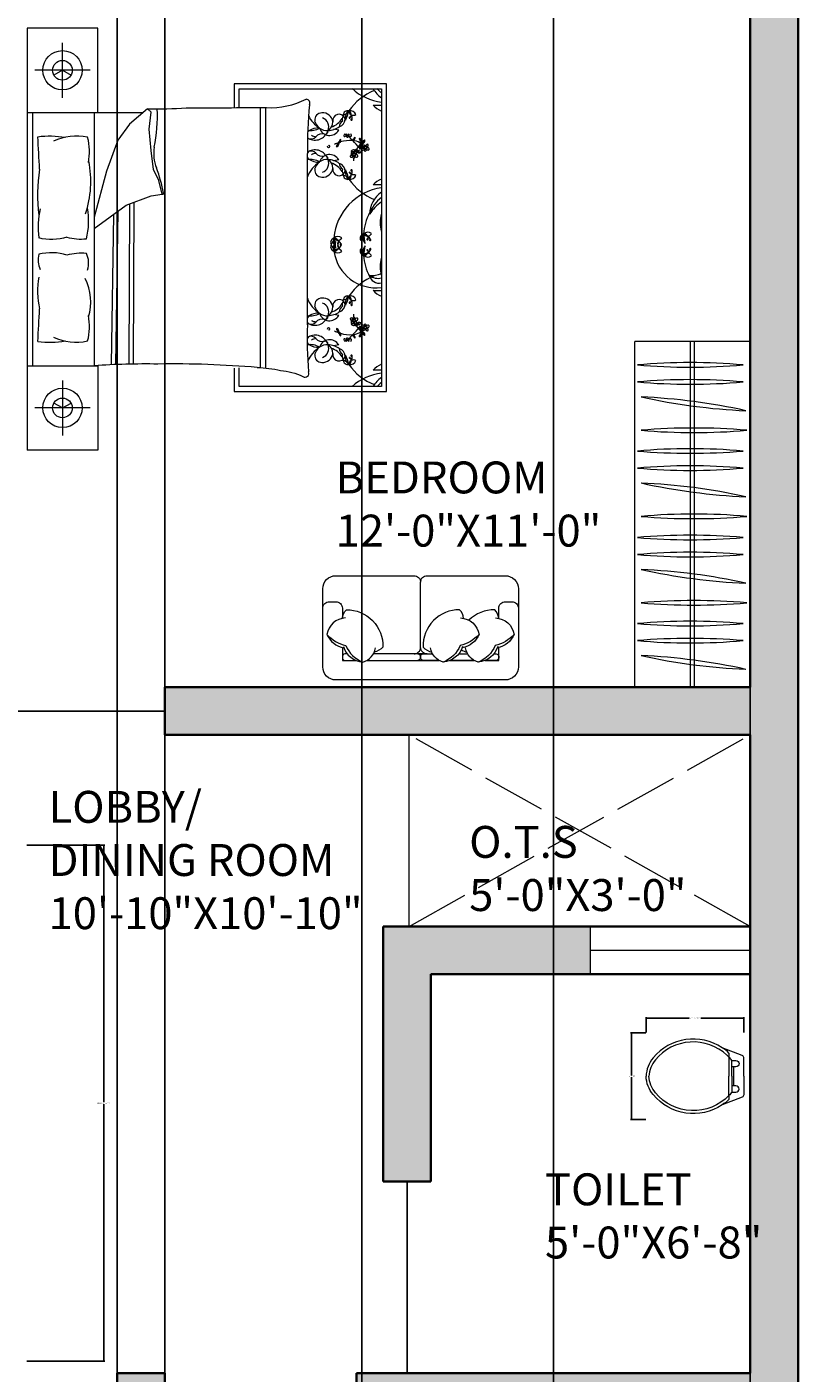
# Model space of a CAD drawing. Units: inches. Extents: x -16 to 587, y -783 to 64.
# Tile 11 of 14: x 92 to 237, y -392 to -138. Entities that reach past the tile are written whole.
import ezdxf

# ---------------------------------------------------------------- set-up
doc = ezdxf.new("R2010")
doc.units = ezdxf.units.IN
doc.header["$MEASUREMENT"] = 0
doc.linetypes.add('ACAD_ISO02W100', pattern=[15, 12, -3])
for name, color, linetype, lineweight in [('A-ANNO-DIMS', 2, 'Continuous', 18), ('A-AREA-IDEN', 7, 'Continuous', 18), ('A-DOOR', 3, 'Continuous', 25), ('A-FLOR-FIXT', 9, 'Continuous', 18), ('A-FLOR-OPEN', 8, 'ACAD_ISO02W100', 13), ('A-FURN', 8, 'Continuous', 18), ('A-GLAZ', 4, 'Continuous', 18), ('A-WALL', 7, 'Continuous', 35), ('A-WALL-PATT', 23, 'Continuous', 13)]:
    doc.layers.add(name, color=color, linetype=linetype, lineweight=lineweight)
doc.styles.get("Standard").update_dxf_attribs({"font": 'arial.ttf'})
doc.dimstyles.get("Standard").update_dxf_attribs({"dimtxt": 0.18, "dimasz": 0.18, "dimexe": 0.18, "dimexo": 0.0625, "dimgap": 0.09, "dimtad": 0, "dimtih": 1, "dimtoh": 1, "dimdec": 0, "dimzin": 0, "dimdsep": 46, "dimlunit": 3, "dimtxsty": 'Standard', "dimcen": 0.09, "dimadec": 0, "dimazin": 0, "dimtfac": 1, "dimtdec": 0, "dimtofl": 0, "dimtmove": 0, "dimatfit": 3, "dimfxl": 1, "dimtolj": 1, "dimtzin": 0, "dimarcsym": 0})

# ---------------------------------------------------------------- blocks, each defined once
blk = doc.blocks.new('BED-DOUBLE-COMPACT')
for p, q in [((0, 79.37), (0, 0)), ((6.61, 66.25), (6.61, 76.62)), ((11.8, 71.43), (1.43, 71.43)), ((38.91, 68.89), (38.91, 64.4)), ((67.5, 68.89), (38.91, 68.89)), ((67.5, 11.03), (67.5, 68.89)), ((39.83, 64.41), (39.83, 67.97)), ((39.83, 67.97), (66.58, 67.97)), ((66.58, 67.97), (66.58, 11.95)), ((0, 63.5), (21.78, 63.5)), ((1.02, 15.87), (1.02, 63.5)), ((12.54, 63.5), (12.54, 15.87)), ((22.61, 64.21), (19.24, 61.31)), ((23.26, 63.56), (22.61, 64.21)), ((22.93, 60.35), (23.26, 63.56)), ((43.86, 15.51), (43.86, 64.41)), ((44.85, 15.44), (44.85, 64.41)), ((19.24, 61.31), (16.99, 58.26)), ((16.99, 58.26), (14.9, 52.47)), ((23.26, 56.33), (22.93, 60.35)), ((58.53, 60.15), (57.63, 60.33)), ((23.74, 52.79), (23.26, 56.33)), ((52.64, 23.57), (52.64, 55.8)), ((58.53, 54.61), (57.63, 54.43)), ((14.9, 52.47), (12.54, 43.82)), ((24.7, 50.7), (23.74, 52.79)), ((25.34, 48.13), (24.7, 50.7)), ((23.26, 47.81), (25.34, 48.13)), ((12.54, 41.69), (18.6, 46.04)), ((18.6, 46.04), (23.26, 47.81)), ((19.15, 16.16), (19.27, 46.3)), ((19.97, 16.15), (20.09, 46.61)), ((15.84, 16.09), (16.24, 44.34)), ((16.65, 16.12), (17.06, 44.94)), ((58.53, 25.32), (57.63, 25.49)), ((58.53, 19.77), (57.63, 19.6)), ((38.91, 15.43), (38.91, 11.03)), ((39.83, 11.95), (39.83, 15.45)), ((6.61, 13.12), (6.61, 2.75)), ((38.91, 11.03), (67.5, 11.03)), ((66.58, 11.95), (39.83, 11.95)), ((11.8, 7.94), (1.43, 7.94))]:
    blk.add_line(p, q)
for points in [[(13.23, 63.5), (13.23, 79.37), (0, 79.37)], [(6.61, 71.43), (5.01, 70.51)], [(6.61, 71.43), (8.22, 70.51)], [(0, 15.87), (13.23, 15.87), (13.23, 0), (0, 0)], [(6.61, 7.94), (5.01, 8.86)], [(6.61, 7.94), (8.22, 8.86)]]:
    blk.add_lwpolyline(points)
for points in [[(29.88, 64.37, -0.001242), (44.94, 64.41, 0.127202), (52.44, 66)], [(1.98, 58.94, -0.074897), (7.16, 58.84, 0.472817)], [(7.45, 40.06, -0.14099), (2.16, 39.9, -0.235245)], [(7.45, 36.67, 0.14099), (2.16, 36.83, 0.235245)], [(1.98, 20.43, 0.074897), (7.16, 20.53, -0.472817)], [(43.23, 15.54, -0.056112), (47.6, 14.96, -0.095341), (51.8, 13.84)]]:
    blk.add_lwpolyline(points, format="xyb")
for centre, radius in [((6.61, 71.43), 3.7), ((6.61, 71.43), 1.85), ((61.41, 55.57), 0.202), ((63.54, 56.89), 0.202), ((61.41, 24.36), 0.202), ((63.54, 23.03), 0.202), ((6.61, 7.94), 3.7), ((6.61, 7.94), 1.85)]:
    blk.add_circle(centre, radius)
for centre, radius, start, end in [((52.39, 65.27), 0.732, 332.6588, 86.02), ((69, 57.96), 10.36, 111.4092, 145.6135), ((67.97, 75.69), 10.36, 228.1144, 262.255), ((69.36, 70.49), 5.05, 209.8884, 236.5383), ((70.3, 72.31), 6.29, 223.5186, 233.6964), ((24.59, 136.98), 72.8, 268.447, 274.1706), ((-5.49, 62.85), 29.95, 348.6608, 2.5481), ((135.26, 56.74), 82.62, 174.3113, 180.6567), ((55.35, 62.08), 1.34, 88.9462, 185.5144), ((55.54, 61.53), 1.9, 7.1143, 95.0551), ((60.24, 62.98), 0.859, 76.272, 177.0484), ((58.93, 64.73), 1.77, 284.7031, 328.6173), ((61.4, 62.48), 1.64, 125.7657, 194.5347), ((53.37, 65.38), 7.25, 332.8176, 347.4827), ((60.69, 62.69), 1.15, 20.9613, 102.2885), ((61.31, 63.84), 0.866, 181.7131, 301.5367), ((58.47, 62.09), 2.62, 2.0648, 41.1598), ((60.05, 63.06), 0.848, 316.2238, 62.3173), ((68.19, 67.66), 4.21, 221.0454, 247.4453), ((65.93, 79.2), 14.34, 266.3481, 272.5919), ((58.23, 65.58), 6.01, 206.7003, 236.3329), ((56.34, 62.49), 2.39, 193.079, 274.7067), ((54.82, 60.79), 1.84, 338.5779, 68.4181), ((55.12, 61.86), 2.31, 305.9599, 357.6409), ((56.28, 64.36), 4.26, 273.4924, 303.7117), ((55.97, 64.33), 3.75, 288.2955, 328.7386), ((58.6, 61.97), 1.19, 19.1312, 189.736), ((58.24, 62.25), 1.49, 285.6955, 4.031), ((60.21, 60.65), 1.58, 128.4175, 173.8338), ((59.89, 62.21), 0.73, 126.7319, 206.0245), ((60.58, 62.55), 0.112, 20.2817, 316.2238), ((60.96, 62.18), 0.129, 168.5166, 2.0648), ((60.9, 62.19), 0.0625, 52.0591, 168.5166), ((-753.35, 15.19), 756.59, 2.85022, 3.31479), ((9.24, 48.82), 10.23, 78.2417, 114.8684), ((1.05, 56.11), 10.64, 348.9631, 14.8961), ((53.52, 59.3), 0.956, 206.442, 225.5483), ((53.52, 59.3), 0.956, 127.675, 149.9707), ((53.23, 63.38), 3.29, 260.8446, 301.1782), ((54.08, 60.83), 2.53, 240.8249, 340.7178), ((53.33, 59.71), 1.19, 246.1646, 318.4347), ((54.66, 57.53), 3.06, 85.2696, 124.215), ((54.54, 61.21), 2.28, 240.0851, 262.564), ((55.44, 57.84), 1.63, 74.8529, 138.4347), ((56.82, 61.14), 1.97, 196.8663, 330.0915), ((55.99, 59.89), 0.493, 254.8529, 12.6959), ((54.66, 57.53), 3.06, 53.6555, 57.2989), ((59.1, 58.03), 0.417, 115.5379, 168.6744), ((57.69, 58.63), 1.25, 329.344, 349.7412), ((56.69, 58.34), 2.24, 352.8698, 1.6736), ((59.65, 59.15), 0.156, 125.0752, 284.7644), ((59.89, 59.21), 0.337, 127.3642, 168.4363), ((59.63, 59.48), 0.486, 277.4968, 341.2737), ((60.01, 59.25), 0.193, 88.1325, 178.8919), ((60.4, 59.04), 0.418, 136.3462, 189.6513), ((60.16, 59), 0.174, 189.6513, 312.3208), ((60.21, 59.49), 0.202, 183.2768, 356.7232), ((60.84, 59.12), 0.662, 164.2829, 186.9148), ((60.06, 59.12), 0.331, 312.3208, 40.2111), ((60.76, 59.49), 0.47, 201.6382, 274.947), ((60.14, 58.85), 0.614, 42.3896, 66.5724), ((66.33, 63.71), 7.54, 217.9541, 226.8459), ((60.58, 59.21), 0.334, 10.9597, 52.2379), ((60.79, 59.18), 0.155, 274.947, 37.5263), ((61.31, 58.3), 0.162, 112.5583, 214.2343), ((61.2, 58.59), 0.381, 265.7131, 351.6568), ((60.87, 58.8), 0.665, 297.3659, 329.344), ((60.36, 59.37), 1.28, 313.6929, 321.7899), ((61.77, 58.5), 0.417, 115.5379, 168.6744), ((60.36, 59.1), 1.25, 329.344, 349.7412), ((59.36, 58.81), 2.24, 352.8698, 1.6736), ((62.5, 58.36), 0.226, 33.0979, 123.1364), ((57.53, 55.18), 5.91, 31.1156, 34.8118), ((62.18, 57.97), 0.611, 2.3172, 70.5201), ((62.39, 58.11), 0.234, 315.7354, 31.1156), ((62.41, 58.04), 0.526, 352.6008, 57.1845), ((62.76, 58.35), 0.611, 291.7087, 3.0299), ((58.4, 61.57), 5.91, 323.6254, 327.3216), ((63.24, 58.19), 0.226, 325.6077, 55.6462), ((30.21, 55.69), 6.46, 168.6608, 203.7384), ((53.52, 55.45), 0.956, 134.4517, 156.771), ((54.08, 53.93), 2.53, 19.2822, 119.1751), ((53.33, 55.05), 1.19, 41.5653, 113.8354), ((54.54, 53.55), 2.28, 97.436, 119.9149), ((55.44, 56.92), 1.63, 221.5653, 285.1471), ((56.64, 57.17), 0.249, 169.5864, 349.5616), ((56.74, 57.15), 0.153, 349.5616, 167.2949), ((60.73, 51.65), 6.57, 110.1059, 116.9968), ((58.53, 57.07), 0.417, 129.5056, 182.6421), ((57.33, 58.03), 1.25, 308.4388, 328.836), ((57.11, 59.05), 2.24, 296.5064, 305.3102), ((57.1, 57.9), 1.28, 336.3901, 344.4871), ((58.48, 57.57), 0.162, 83.9457, 185.6216), ((57.84, 57.73), 0.665, 328.836, 0.8141), ((58.18, 57.53), 0.381, 306.5232, 32.4668), ((58.64, 57.83), 0.162, 112.5583, 214.2343), ((58.53, 58.12), 0.381, 265.7131, 351.6568), ((58.2, 58.33), 0.665, 297.3659, 329.344), ((57.69, 58.9), 1.28, 313.6929, 321.7899), ((60.73, 51.65), 6.57, 86.1723, 106.4158), ((61.11, 57.11), 0.921, 253.6301, 325.4631), ((61.37, 55.83), 0.652, 82.0748, 142.6895), ((61.29, 56.73), 0.669, 228.342, 274.9894), ((61.05, 55.82), 0.198, 138.2946, 276.2474), ((61.13, 55.79), 0.276, 358.5719, 143.8954), ((61.29, 56.01), 0.278, 208.8493, 269.9355), ((61.05, 55.94), 0.318, 274.2123, 318.1587), ((60.9, 54.92), 3.3, 60.7959, 85.244), ((53.88, 50.18), 10.84, 37.8256, 47.7588), ((61.31, 56.62), 0.56, 273.8774, 357.1501), ((62.02, 55.62), 0.637, 121.9501, 165.2442), ((61.53, 57.02), 0.542, 262.0748, 308.2393), ((61.58, 55.87), 0.134, 262.868, 7.094), ((61.56, 55.98), 0.399, 278.5614, 22.5914), ((65.28, 54.59), 3.95, 156.1523, 156.9499), ((61.79, 55.99), 0.2, 44.3732, 121.9501), ((62.4, 56.46), 0.56, 181.4625, 249.4747), ((65.28, 54.59), 3.95, 130.182, 149.456), ((62.31, 56.9), 0.542, 215.1128, 261.2773), ((62.74, 56.87), 0.921, 197.889, 269.722), ((62.46, 56.56), 0.669, 248.3627, 295.0101), ((62.13, 55.72), 0.652, 20.6625, 81.2773), ((63.1, 56.84), 0.652, 139.3812, 199.9959), ((61.88, 57.31), 0.921, 310.9365, 22.7695), ((62.31, 57.26), 0.669, 285.6484, 332.2957), ((62.68, 57.82), 0.176, 135.7354, 318.1297), ((62.19, 57.61), 0.542, 319.3812, 5.5456), ((62.81, 57.82), 0.176, 68.2452, 250.6395), ((64.29, 54.51), 3.52, 111.7087, 116.2181), ((60.9, 54.92), 3.3, 47.5083, 55.9967), ((62.91, 58.16), 0.526, 252.8042, 349.6943), ((62.41, 57.22), 0.56, 331.1838, 51.6792), ((62.98, 56.55), 0.156, 125.0752, 284.7644), ((62.97, 58.2), 0.234, 248.2452, 323.6254), ((63.22, 56.61), 0.337, 93.635, 168.4363), ((63.18, 57.14), 0.198, 138.2946, 276.2474), ((62.96, 56.88), 0.486, 277.4968, 341.2737), ((63.26, 57.11), 0.276, 358.5719, 143.8954), ((63.35, 56.65), 0.193, 88.1325, 178.8919), ((63.42, 57.33), 0.278, 208.8493, 269.9355), ((63.18, 57.26), 0.318, 274.2123, 318.1587), ((63.73, 56.45), 0.418, 136.3462, 189.6513), ((63.49, 56.41), 0.174, 189.6513, 312.3208), ((64.17, 56.53), 0.662, 164.2829, 186.9148), ((64.15, 56.94), 0.637, 121.9501, 165.2442), ((63.39, 56.52), 0.331, 312.3208, 40.2111), ((64.09, 56.9), 0.47, 201.6382, 274.947), ((63.71, 57.19), 0.134, 262.868, 7.094), ((63.47, 56.25), 0.614, 42.3896, 66.5724), ((63.69, 57.3), 0.399, 278.5614, 22.5914), ((63.91, 56.61), 0.334, 10.9597, 118.7804), ((63.92, 57.31), 0.2, 44.3732, 121.9501), ((64.12, 56.58), 0.155, 274.947, 37.5263), ((-6.51, 50.51), 18.45, 340.7385, 11.9603), ((53.52, 55.45), 0.956, 203.2856, 232.325), ((53.23, 51.38), 3.29, 58.8218, 100.2867), ((58.23, 49.18), 6.01, 123.6671, 158.5059), ((54.66, 57.23), 3.06, 235.785, 274.7304), ((56.34, 52.27), 2.39, 85.2933, 166.921), ((56.82, 53.62), 1.97, 29.9085, 163.1337), ((54.82, 53.97), 1.84, 291.5819, 21.4221), ((55.99, 54.87), 0.493, 347.3041, 105.1471), ((54.66, 57.23), 3.06, 302.7011, 306.3445), ((55.12, 52.9), 2.31, 2.3591, 54.0401), ((56.28, 50.39), 4.26, 56.2883, 86.5076), ((55.97, 50.43), 3.75, 31.2614, 71.7045), ((60.21, 54.11), 1.58, 186.1662, 231.5825), ((58.24, 52.5), 1.49, 355.969, 74.3045), ((60.85, 55.23), 0.156, 125.0752, 284.7644), ((61.09, 55.29), 0.337, 93.635, 168.4363), ((60.83, 55.56), 0.486, 277.4968, 341.2737), ((61.22, 55.33), 0.193, 88.1325, 178.8919), ((61.6, 55.13), 0.418, 136.3462, 189.6513), ((61.36, 55.09), 0.174, 189.6513, 312.3208), ((65.28, 54.59), 3.95, 175.2415, 182.8929), ((62.04, 55.21), 0.662, 164.2829, 186.9148), ((61.26, 55.2), 0.331, 312.3208, 40.2111), ((61.96, 55.57), 0.47, 201.6382, 274.947), ((61.34, 54.93), 0.614, 42.3896, 66.5724), ((61.78, 55.29), 0.334, 10.9597, 118.7804), ((61.99, 55.26), 0.155, 274.947, 37.5263), ((30.7, 48.06), 28.79, 170.503, 187.7804), ((-4.65, 42.62), 30.78, 10.6617, 19.8806), ((55.35, 52.68), 1.34, 174.4856, 271.0538), ((55.54, 53.23), 1.9, 264.9449, 352.8857), ((58.6, 52.79), 1.19, 170.264, 340.8688), ((59.89, 52.54), 0.73, 153.9755, 233.2681), ((60.24, 51.78), 0.859, 182.9516, 283.728), ((58.93, 50.02), 1.77, 31.3827, 75.2969), ((61.4, 52.28), 1.64, 165.4653, 234.2343), ((53.37, 49.37), 7.25, 12.5173, 27.1824), ((58.47, 52.67), 2.62, 318.8402, 357.9352), ((60.05, 51.7), 0.848, 297.6827, 43.7762), ((61.31, 50.92), 0.866, 58.4633, 178.2869), ((60.69, 52.07), 1.15, 257.7115, 339.0387), ((69, 56.8), 10.36, 214.3865, 248.5908), ((60.54, 52.19), 0.0676, 43.7729, 339.7333), ((60.96, 52.58), 0.129, 357.9352, 191.4834), ((60.9, 52.57), 0.0625, 191.4834, 307.9409), ((68.19, 47.1), 4.21, 112.5547, 138.9546), ((25.41, 48.31), 0.192, 250.2464, 1.1377), ((67.97, 39.07), 10.36, 97.745, 175.5377), ((69.36, 44.27), 5.05, 123.4617, 178.728), ((65.93, 35.55), 14.34, 87.4081, 93.6519), ((70.3, 42.45), 6.29, 126.3036, 162.1496), ((72.07, 39.14), 9.36, 125.947, 145.9877), ((16.15, 41.98), 14.14, 166.04, 188.4751), ((-2.48, 43.04), 14, 346.3762, 10.1383), ((73.53, 39.86), 10.36, 152.5854, 175.5377), ((72.03, 42.76), 5.7, 162.9798, 196.4569), ((63.43, 39.84), 0.859, 106.1963, 206.9726), ((61.42, 40.71), 1.77, 314.6273, 358.5415), ((64.69, 39.99), 1.64, 155.6899, 224.4589), ((63.97, 39.82), 1.15, 50.8855, 132.2127), ((63.93, 41.12), 0.866, 211.6373, 331.4609), ((62.34, 38.19), 2.62, 31.989, 71.0841), ((56.27, 38.5), 7.25, 2.7418, 17.407), ((63.23, 39.82), 0.848, 346.148, 92.2415), ((74.96, 40.5), 8.43, 174.3643, 175.6213), ((80.74, 36.06), 15.06, 160.0972, 160.2783), ((10.1, 49.41), 9.72, 254.1707, 275.9871), ((57.88, 39.05), 0.859, 106.1963, 206.9726), ((57.88, 38.23), 0.859, 153.0274, 253.8037), ((55.87, 39.92), 1.77, 314.6273, 358.5415), ((55.87, 37.36), 1.77, 1.4585, 45.3727), ((59.14, 39.2), 1.64, 155.6899, 224.4589), ((59.14, 38.08), 1.64, 135.5411, 204.3101), ((58.41, 39.02), 1.15, 50.8855, 132.2127), ((58.38, 40.33), 0.866, 211.6373, 331.4609), ((50.72, 37.7), 7.25, 2.7418, 17.407), ((57.67, 39.03), 0.848, 346.148, 92.2415), ((56.79, 37.39), 2.62, 31.989, 71.0841), ((50.72, 39.57), 7.25, 342.593, 357.2582), ((56.79, 39.88), 2.62, 288.9159, 328.011), ((57.67, 38.25), 0.848, 267.7585, 13.852), ((58.39, 38.85), 0.112, 50.0755, 346.148), ((58.35, 38.44), 0.0676, 13.9791, 309.8091), ((58.91, 38.71), 0.129, 198.4408, 31.989), ((58.84, 38.69), 0.0625, 81.9833, 198.4408), ((58.91, 38.56), 0.129, 328.011, 161.5592), ((58.84, 38.58), 0.0625, 161.5592, 278.0167), ((64.69, 37.28), 1.64, 135.5411, 204.3101), ((56.27, 38.78), 7.25, 342.593, 357.2582), ((63.94, 39.64), 0.112, 50.0755, 346.148), ((64.39, 39.49), 0.0625, 81.9833, 198.4408), ((64.46, 39.51), 0.129, 198.4408, 31.989), ((5.94, 35.74), 3.93, 163.8974, 206.6563), ((10.1, 27.31), 9.72, 84.0129, 105.8293), ((7.31, 35.21), 4.21, 341.4593, 24.9817), ((58.38, 36.95), 0.866, 28.5391, 148.3627), ((58.41, 38.25), 1.15, 227.7873, 309.1145), ((65.58, 38.54), 8.02, 188.1803, 277.1364), ((63.43, 37.44), 0.859, 153.0274, 253.8037), ((61.42, 36.56), 1.77, 1.4585, 45.3727), ((62.34, 39.09), 2.62, 288.9159, 328.011), ((63.23, 37.46), 0.848, 267.7585, 13.852), ((63.93, 36.16), 0.866, 28.5391, 148.3627), ((63.97, 37.46), 1.15, 227.7873, 309.1145), ((73.53, 37.42), 10.36, 184.4623, 207.4146), ((63.9, 37.64), 0.0676, 13.9791, 309.8091), ((64.39, 37.79), 0.0625, 161.5592, 278.0167), ((64.46, 37.77), 0.129, 328.011, 161.5592), ((72.03, 34.52), 5.7, 163.5431, 197.0202), ((74.96, 36.78), 8.43, 184.3787, 185.6357), ((80.74, 41.21), 15.06, 199.7217, 199.9028), ((64.85, 37.51), 4.64, 263.3805, 291.883), ((15.87, 29.85), 13.95, 168.8159, 193.6573), ((1.83, 27.85), 10.1, 343.8254, 26.1239), ((69, 23.12), 10.36, 111.4092, 145.6135), ((66.14, 33.25), 1.86, 190.9261, 283.6102), ((65.88, 34.65), 2.35, 228.0951, 287.1391), ((58.23, 30.75), 6.01, 201.4941, 236.3329), ((55.35, 27.25), 1.34, 88.9462, 185.5144), ((55.54, 26.7), 1.9, 7.1143, 95.0551), ((58.6, 27.13), 1.19, 19.1312, 189.736), ((59.89, 27.38), 0.73, 126.7319, 206.0245), ((60.24, 28.14), 0.859, 76.272, 177.0484), ((58.93, 29.9), 1.77, 284.7031, 328.6173), ((61.4, 27.65), 1.64, 125.7657, 194.5347), ((53.37, 30.55), 7.25, 332.8176, 347.4827), ((60.69, 27.85), 1.15, 20.9613, 102.2885), ((60.05, 28.23), 0.848, 316.2238, 62.3173), ((58.47, 27.25), 2.62, 2.0648, 41.1598), ((61.31, 29), 0.866, 181.7131, 301.5367), ((65.93, 44.37), 14.34, 266.3481, 272.5919), ((68.19, 32.83), 4.21, 221.0454, 247.4453), ((-753.35, 64.18), 756.59, 356.68521, 357.14978), ((53.23, 28.54), 3.29, 259.7133, 301.1782), ((54.66, 22.7), 3.06, 85.2696, 124.215), ((56.34, 27.66), 2.39, 193.079, 274.7067), ((56.82, 26.3), 1.97, 196.8663, 330.0915), ((54.82, 25.95), 1.84, 338.5779, 68.4181), ((55.12, 27.03), 2.31, 305.9599, 357.6409), ((56.28, 29.53), 4.26, 273.4924, 303.7117), ((55.97, 29.5), 3.75, 288.2955, 328.7386), ((58.24, 27.42), 1.49, 285.6955, 4.031), ((60.21, 25.82), 1.58, 128.4175, 173.8338), ((60.58, 27.72), 0.112, 20.2817, 316.2238), ((60.96, 27.34), 0.129, 168.5166, 2.0648), ((60.9, 27.35), 0.0625, 52.0591, 168.5166), ((65.28, 25.34), 3.95, 177.1071, 184.7585), ((1.05, 23.26), 10.64, 345.1039, 11.0369), ((129.84, 21.14), 77.23, 178.1965, 184.7598), ((53.52, 24.47), 0.956, 127.675, 156.7144), ((53.52, 24.47), 0.956, 203.2856, 225.5483), ((54.08, 26), 2.53, 240.8249, 340.7178), ((53.33, 24.87), 1.19, 246.1646, 318.4347), ((54.54, 26.38), 2.28, 240.0851, 262.564), ((55.44, 23.01), 1.63, 74.8529, 138.4347), ((55.99, 25.05), 0.493, 254.8529, 12.6959), ((54.66, 22.7), 3.06, 53.6555, 57.2989), ((56.64, 22.76), 0.249, 10.4384, 190.4136), ((56.74, 22.77), 0.153, 192.7051, 10.4384), ((57.33, 21.89), 1.25, 31.164, 51.5612), ((58.53, 22.86), 0.417, 177.3579, 230.4944), ((57.11, 20.87), 2.24, 54.6898, 63.4936), ((60.85, 24.7), 0.156, 75.2356, 234.9248), ((61.09, 24.64), 0.337, 191.5637, 266.365), ((61.05, 24.1), 0.198, 83.7526, 221.7054), ((61.29, 23.19), 0.669, 85.0106, 131.658), ((61.11, 22.81), 0.921, 34.5369, 106.3699), ((61.37, 24.09), 0.652, 217.3105, 277.9252), ((60.83, 24.37), 0.486, 18.7263, 82.5032), ((61.13, 24.13), 0.276, 216.1046, 1.4281), ((61.22, 24.59), 0.193, 181.1081, 271.8675), ((61.29, 23.92), 0.278, 90.0645, 151.1507), ((61.05, 23.98), 0.318, 41.8413, 85.7877), ((53.88, 29.74), 10.84, 312.2412, 322.1744), ((61.36, 24.84), 0.174, 47.6792, 170.3487), ((61.6, 24.8), 0.418, 170.3487, 223.6538), ((61.31, 23.3), 0.56, 2.8499, 86.1226), ((62.04, 24.72), 0.662, 173.0852, 195.7171), ((62.02, 24.3), 0.637, 194.7558, 238.0499), ((61.53, 22.91), 0.542, 51.7607, 97.9252), ((61.26, 24.72), 0.331, 319.7889, 47.6792), ((61.96, 24.35), 0.47, 85.053, 158.3618), ((61.58, 24.06), 0.134, 352.906, 97.132), ((61.34, 24.99), 0.614, 293.4276, 317.6104), ((61.78, 24.63), 0.334, 241.2196, 349.0403), ((61.56, 23.94), 0.399, 337.4086, 81.4386), ((65.28, 25.34), 3.95, 203.0501, 203.8477), ((61.79, 23.93), 0.2, 238.0499, 315.6268), ((62.4, 23.46), 0.56, 110.5253, 178.5375), ((62.74, 23.05), 0.921, 90.278, 162.111), ((62.31, 23.02), 0.542, 98.7227, 144.8872), ((65.28, 25.34), 3.95, 210.544, 229.818), ((61.99, 24.66), 0.155, 322.4737, 85.053), ((62.46, 23.36), 0.669, 64.9899, 111.6373), ((62.13, 24.2), 0.652, 278.7227, 339.3375), ((63.1, 23.09), 0.652, 160.0041, 220.6188), ((61.88, 22.61), 0.921, 337.2305, 49.0635), ((62.31, 22.66), 0.669, 27.7043, 74.3516), ((62.41, 22.71), 0.56, 308.3208, 28.8162), ((62.98, 23.37), 0.156, 75.2356, 234.9248), ((63.22, 23.31), 0.337, 191.5637, 266.365), ((63.18, 22.78), 0.198, 83.7526, 221.7054), ((62.96, 23.04), 0.486, 18.7263, 82.5032), ((63.26, 22.81), 0.276, 216.1046, 1.4281), ((63.35, 23.27), 0.193, 181.1081, 271.8675), ((63.42, 22.59), 0.278, 90.0645, 151.1507), ((63.18, 22.66), 0.318, 41.8413, 85.7877), ((63.49, 23.52), 0.174, 47.6792, 170.3487), ((63.73, 23.47), 0.418, 170.3487, 223.6538), ((64.17, 23.4), 0.662, 173.0852, 195.7171), ((64.15, 22.98), 0.637, 194.7558, 238.0499), ((63.39, 23.4), 0.331, 319.7889, 47.6792), ((64.09, 23.03), 0.47, 85.053, 158.3618), ((63.71, 22.74), 0.134, 352.906, 97.132), ((63.47, 23.67), 0.614, 293.4276, 317.6104), ((63.91, 23.31), 0.334, 241.2196, 349.0403), ((63.69, 22.62), 0.399, 337.4086, 81.4386), ((64.12, 23.34), 0.155, 322.4737, 85.053), ((9.24, 30.54), 10.23, 245.1316, 281.7583), ((53.52, 20.62), 0.956, 134.4517, 163.3657), ((53.52, 20.62), 0.956, 197.4186, 232.325), ((54.08, 19.09), 2.53, 19.2822, 119.1751), ((53.33, 20.22), 1.19, 41.5653, 113.8354), ((54.54, 18.71), 2.28, 97.436, 119.9149), ((55.44, 22.08), 1.63, 221.5653, 285.1471), ((56.82, 18.79), 1.97, 29.9085, 163.1337), ((55.99, 20.04), 0.493, 347.3041, 105.1471), ((60.73, 28.27), 6.57, 243.0032, 249.8941), ((57.1, 22.02), 1.28, 15.5129, 23.6099), ((58.48, 22.35), 0.162, 174.3784, 276.0543), ((58.18, 22.39), 0.381, 327.5332, 53.4768), ((57.84, 22.2), 0.665, 359.1859, 31.164), ((58.64, 22.1), 0.162, 145.7657, 247.4417), ((58.53, 21.81), 0.381, 8.3432, 94.2869), ((58.2, 21.6), 0.665, 30.656, 62.6341), ((57.69, 21.03), 1.28, 38.2101, 46.3071), ((59.1, 21.9), 0.417, 191.3256, 244.4621), ((57.69, 21.3), 1.25, 10.2588, 30.656), ((60.73, 28.27), 6.57, 253.5842, 273.8277), ((56.69, 21.59), 2.24, 358.3264, 7.1302), ((59.65, 20.78), 0.156, 75.2356, 234.9248), ((59.89, 20.72), 0.337, 191.5637, 232.6358), ((59.63, 20.45), 0.486, 18.7263, 82.5032), ((60.01, 20.67), 0.193, 181.1081, 271.8675), ((60.16, 20.92), 0.174, 47.6792, 170.3487), ((60.4, 20.88), 0.418, 170.3487, 223.6538), ((60.21, 20.44), 0.202, 3.2768, 176.7232), ((60.84, 20.8), 0.662, 173.0852, 195.7171), ((60.06, 20.8), 0.331, 319.7889, 47.6792), ((60.76, 20.43), 0.47, 85.053, 158.3618), ((66.33, 16.22), 7.54, 133.1541, 142.0459), ((60.14, 21.07), 0.614, 293.4276, 317.6104), ((60.58, 20.71), 0.334, 307.7621, 349.0403), ((60.79, 20.74), 0.155, 322.4737, 85.053), ((61.31, 21.62), 0.162, 145.7657, 247.4417), ((60.9, 25), 3.3, 274.756, 299.2041), ((61.2, 21.33), 0.381, 8.3432, 94.2869), ((60.87, 21.12), 0.665, 30.656, 62.6341), ((60.36, 20.55), 1.28, 38.2101, 46.3071), ((61.77, 21.42), 0.417, 191.3256, 244.4621), ((60.36, 20.82), 1.25, 10.2588, 30.656), ((59.36, 21.11), 2.24, 358.3264, 7.1302), ((62.18, 21.95), 0.611, 289.4799, 357.6828), ((57.53, 24.75), 5.91, 325.1882, 328.8844), ((62.5, 21.56), 0.226, 236.8636, 326.9021), ((62.68, 22.1), 0.176, 41.8703, 224.2646), ((62.39, 21.82), 0.234, 328.8844, 44.2646), ((62.19, 22.31), 0.542, 354.4544, 40.6188), ((62.81, 22.1), 0.176, 109.3605, 291.7548), ((62.41, 21.88), 0.526, 302.8155, 7.3992), ((64.29, 25.42), 3.52, 243.7819, 248.2913), ((60.9, 25), 3.3, 304.0033, 312.4917), ((62.91, 21.76), 0.526, 10.3057, 107.1958), ((62.97, 21.72), 0.234, 36.3746, 111.7548), ((62.76, 21.58), 0.611, 356.9701, 68.2913), ((58.4, 18.36), 5.91, 32.6784, 36.3746), ((63.24, 21.73), 0.226, 304.3538, 34.3923), ((63.92, 22.61), 0.2, 238.0499, 315.6268), ((53.23, 16.55), 3.29, 58.8218, 100.751), ((58.23, 14.34), 6.01, 123.6671, 156.3547), ((54.66, 22.39), 3.06, 235.785, 274.7304), ((56.34, 17.43), 2.39, 85.2933, 166.921), ((55.35, 17.84), 1.34, 174.4856, 271.0538), ((55.54, 18.39), 1.9, 264.9449, 352.8857), ((54.82, 19.14), 1.84, 291.5819, 21.4221), ((54.66, 22.39), 3.06, 302.7011, 306.3445), ((55.12, 18.06), 2.31, 2.3591, 54.0401), ((56.28, 15.56), 4.26, 56.2883, 86.5076), ((55.97, 15.59), 3.75, 31.2614, 71.7045), ((58.6, 17.96), 1.19, 170.264, 340.8688), ((58.24, 17.67), 1.49, 355.969, 74.3045), ((60.21, 19.27), 1.58, 186.1662, 231.5825), ((59.89, 17.71), 0.73, 153.9755, 233.2681), ((61.4, 17.44), 1.64, 165.4653, 234.2343), ((53.37, 14.54), 7.25, 12.5173, 27.1824), ((58.47, 17.84), 2.62, 318.8402, 357.9352), ((60.96, 17.75), 0.129, 357.9352, 191.4834), ((60.9, 17.73), 0.0625, 191.4834, 307.9409), ((22.24, -126.41), 142.61, 89.0718, 93.9), ((27.43, -169.82), 186.03, 85.1265, 90.8855), ((58.93, 15.19), 1.77, 31.3827, 75.2969), ((60.24, 16.95), 0.859, 182.9516, 283.728), ((60.05, 16.86), 0.848, 297.6827, 43.7762), ((61.31, 16.09), 0.866, 58.4633, 178.2869), ((60.69, 17.24), 1.15, 257.7115, 339.0387), ((69, 21.97), 10.36, 214.3865, 248.5908), ((60.54, 17.36), 0.0676, 43.7729, 339.7333), ((68.19, 12.26), 4.21, 112.5547, 138.9546), ((52.21, 14.44), 0.723, 236.1736, 23.4781), ((67.97, 4.23), 10.36, 97.745, 131.8856), ((69.36, 9.43), 5.05, 123.4617, 150.1116), ((65.93, 0.72), 14.34, 87.4081, 93.6519), ((70.3, 7.62), 6.29, 126.3036, 136.4814)]:
    blk.add_arc(centre, radius, start, end)
blk = doc.blocks.new('WARDROBE')
for p, q in [((0, 0), (0, 65.01)), ((21.67, 65.01), (0, 65.01)), ((10.47, 0), (10.47, 65.01)), ((11.19, 0), (11.19, 65.01)), ((21.67, 0), (21.67, 65.01)), ((21.67, 0), (0, 0))]:
    blk.add_line(p, q)
for centre, start, end in [((10.4, -52.98), 85.0028, 94.9972), ((10.4, 174.18), 265.0028, 274.9972), ((10.4, -56.19), 85.0028, 94.9972), ((10.4, 170.97), 265.0028, 274.9972), ((25.83, 165.89), 257.508, 267.5023), ((-3.8, -59.33), 77.508, 87.5023), ((11.1, -65.28), 85.0028, 94.9972), ((11.1, 161.88), 265.0028, 274.9972), ((10.4, -69.18), 85.0028, 94.9972), ((10.4, 157.98), 265.0028, 274.9972), ((10.4, -72.39), 85.0028, 94.9972), ((10.4, 154.77), 265.0028, 274.9972), ((25.83, 149.7), 257.508, 267.5023), ((-3.8, -75.52), 77.508, 87.5023), ((11.1, -81.47), 85.0028, 94.9972), ((11.1, 145.69), 265.0028, 274.9972), ((10.4, -85.44), 85.0028, 94.9972), ((10.4, 141.72), 265.0028, 274.9972), ((10.4, -88.65), 85.0028, 94.9972), ((10.4, 138.51), 265.0028, 274.9972), ((-3.8, -91.78), 77.508, 87.5023), ((25.83, 133.44), 257.508, 267.5023), ((11.1, -97.73), 85.0028, 94.9972), ((11.1, 129.43), 265.0028, 274.9972), ((10.4, -101.63), 85.0028, 94.9972), ((10.4, 125.53), 265.0028, 274.9972), ((10.4, -104.84), 85.0028, 94.9972), ((10.4, 122.32), 265.0028, 274.9972), ((-3.8, -107.97), 77.508, 87.5023), ((25.83, 117.25), 257.508, 267.5023)]:
    blk.add_arc(centre, 114.01, start, end)
blk = doc.blocks.new('WC-PLAN')
for p, q in [((15.58, 11.39), (15.58, 10.62)), ((15.58, 10.62), (15.58, 7.01)), ((15.58, 3.4), (15.58, 7.01)), ((15.58, 3.4), (15.58, 2.63))]:
    blk.add_line(p, q)
for points in [[(14.32, 12.39, 0.383919), (1.32, 10.46, 0.163732), (0, 7.01, 0.359733)], [(15.2, 10.99, 0.431639), (1.75, 10.11, 0.162618), (0.55, 7.01, 0.470877)], [(15.58, 11.39, 0.040937), (14.32, 12.39, 0.163732)], [(18.36, 7.01), (18.36, 10.52, 0.31031), (18.06, 10.95), (14.32, 12.39, 0.209071)], [(15.58, 10.62, 0.014165), (15.2, 10.99, 0.162618)], [(16.13, 9.99, 0.022712), (15.58, 10.62, 0.162618)], [(16.13, 7.01), (16.13, 9.99, 0.022712)], [(16.13, 9.99), (16.9, 9.99, -1), (16.9, 8.82), (16.5, 8.82)], [(14.32, 1.64, -0.383919), (1.32, 3.56, -0.163732), (0, 7.01, -0.359733)], [(15.58, 3.4, -0.448546), (1.75, 3.91, -0.162618), (0.55, 7.01, -0.470877)], [(18.36, 7.01), (18.36, 3.51, -0.31031), (18.06, 3.08), (14.32, 1.64, -0.209071)], [(16.13, 7.01), (16.13, 4.03, -0.476108)], [(16.13, 4.03), (16.9, 4.03, 1), (16.9, 5.21), (16.5, 5.21)], [(15.58, 2.63, -0.040937), (14.32, 1.64, -0.163732)], [(16.13, 4.03, -0.022712), (15.58, 3.4, -0.162618)]]:
    blk.add_lwpolyline(points, format="xyb")
for points in [[(16.5, 8.82), (16.13, 8.82)], [(16.5, 5.21), (16.5, 8.82)], [(16.5, 5.21), (16.13, 5.21)]]:
    blk.add_lwpolyline(points)
blk = doc.blocks.new('*D30')
at = {"layer": 'A-ANNO-DIMS', "color": 0, "lineweight": -2, "transparency": 16777216}
for p, q in [((208.51, -327.52), (208.51, -324.65)), ((208.69, -324.83), (216.59, -324.83)), ((226.69, -324.83), (218.79, -324.83)), ((226.87, -327.52), (226.87, -324.65))]:
    blk.add_line(p, q, dxfattribs=at)
at = {"layer": 'A-ANNO-DIMS', "color": 0, "transparency": 16777216}
for points in [[(208.69, -324.8), (208.69, -324.86), (208.51, -324.83)], [(226.69, -324.8), (226.69, -324.86), (226.87, -324.83)]]:
    blk.add_solid(points, dxfattribs=at)
at = {"layer": 'Defpoints', "color": 0, "transparency": 16777216}
for p in [(226.87, -324.83), (208.51, -327.58), (226.87, -327.58)]:
    blk.add_point(p, dxfattribs=at)
at = {"layer": 'A-ANNO-DIMS', "color": 0, "transparency": 16777216, "insert": (217.69, -324.83), "char_height": 0.18, "attachment_point": 5}
blk.add_mtext('\\A1;WC 1\'-6 1/2" TYP.', dxfattribs=at)
blk = doc.blocks.new('*D31')
at = {"layer": 'A-ANNO-DIMS', "color": 0, "lineweight": -2, "transparency": 16777216}
for p, q in [((208.45, -327.58), (205.58, -327.58)), ((205.76, -327.76), (205.76, -335.56)), ((205.76, -343.71), (205.76, -335.92)), ((208.45, -343.89), (205.58, -343.89))]:
    blk.add_line(p, q, dxfattribs=at)
at = {"layer": 'A-ANNO-DIMS', "color": 0, "transparency": 16777216}
for points in [[(205.73, -327.76), (205.79, -327.76), (205.76, -327.58)], [(205.73, -343.71), (205.79, -343.71), (205.76, -343.89)]]:
    blk.add_solid(points, dxfattribs=at)
at = {"layer": 'Defpoints', "color": 0, "transparency": 16777216}
for p in [(205.76, -327.58), (208.51, -327.58), (208.51, -343.89)]:
    blk.add_point(p, dxfattribs=at)
at = {"layer": 'A-ANNO-DIMS', "color": 0, "transparency": 16777216, "insert": (205.76, -335.74), "char_height": 0.18, "attachment_point": 5}
blk.add_mtext('\\A1;1\'-4 1/2" TYP.', dxfattribs=at)
blk = doc.blocks.new('*D36')
at = {"layer": 'A-ANNO-DIMS', "color": 0, "lineweight": -2, "transparency": 16777216}
for p, q in [((92.12, -292.26), (106.79, -292.26)), ((106.61, -292.44), (106.61, -340.6)), ((106.61, -389.13), (106.61, -340.97)), ((92.12, -389.31), (106.79, -389.31))]:
    blk.add_line(p, q, dxfattribs=at)
at = {"layer": 'A-ANNO-DIMS', "color": 0, "transparency": 16777216}
for points in [[(106.58, -292.44), (106.64, -292.44), (106.61, -292.26)], [(106.58, -389.13), (106.64, -389.13), (106.61, -389.31)]]:
    blk.add_solid(points, dxfattribs=at)
at = {"layer": 'Defpoints', "color": 0, "transparency": 16777216}
for p in [(92.05, -292.26), (106.61, -292.26), (92.05, -389.31)]:
    blk.add_point(p, dxfattribs=at)
at = {"layer": 'A-ANNO-DIMS', "color": 0, "transparency": 16777216, "insert": (106.61, -340.78), "char_height": 0.18, "attachment_point": 5}
blk.add_mtext('\\A1;DINING SET 8\'-1" TYP.', dxfattribs=at)
blk = doc.blocks.new('*D56')
at = {"layer": 'A-ANNO-DIMS', "color": 0, "lineweight": -2, "transparency": 16777216}
for p, q in [((118.08, -728.49), (118.08, 63.78)), ((118.26, 63.6), (172.75, 63.6)), ((227.9, 63.6), (173.41, 63.6)), ((228.08, -728.49), (228.08, 63.78))]:
    blk.add_line(p, q, dxfattribs=at)
at = {"layer": 'A-ANNO-DIMS', "color": 0, "transparency": 16777216}
for points in [[(118.26, 63.63), (118.26, 63.57), (118.08, 63.6)], [(227.9, 63.63), (227.9, 63.57), (228.08, 63.6)]]:
    blk.add_solid(points, dxfattribs=at)
at = {"layer": 'Defpoints', "color": 0, "transparency": 16777216}
for p in [(228.08, 63.6), (118.08, -728.55), (228.08, -728.55)]:
    blk.add_point(p, dxfattribs=at)
at = {"layer": 'A-ANNO-DIMS', "color": 0, "transparency": 16777216, "insert": (173.08, 63.6), "char_height": 0.18, "attachment_point": 5}
blk.add_mtext('\\A1;9\'-2"', dxfattribs=at)
blk = doc.blocks.new('*D57')
at = {"layer": 'A-ANNO-DIMS', "color": 0, "lineweight": -2, "transparency": 16777216}
for p, q in [((155.08, -534.49), (155.08, 63.78)), ((155.26, 63.6), (172.75, 63.6)), ((190.9, 63.6), (173.41, 63.6)), ((191.08, -534.49), (191.08, 63.78))]:
    blk.add_line(p, q, dxfattribs=at)
at = {"layer": 'A-ANNO-DIMS', "color": 0, "transparency": 16777216}
for points in [[(155.26, 63.63), (155.26, 63.57), (155.08, 63.6)], [(190.9, 63.63), (190.9, 63.57), (191.08, 63.6)]]:
    blk.add_solid(points, dxfattribs=at)
at = {"layer": 'Defpoints', "color": 0, "transparency": 16777216}
for p in [(191.08, 63.6), (155.08, -534.55), (191.08, -534.55)]:
    blk.add_point(p, dxfattribs=at)
at = {"layer": 'A-ANNO-DIMS', "color": 0, "transparency": 16777216, "insert": (173.08, 63.6), "char_height": 0.18, "attachment_point": 5}
blk.add_mtext('\\A1;3\'-0"', dxfattribs=at)
blk = doc.blocks.new('*D58')
at = {"layer": 'A-ANNO-DIMS', "color": 0, "lineweight": -2, "transparency": 16777216}
for p, q in [((73.08, -663.49), (73.08, 63.78)), ((73.26, 63.6), (90.75, 63.6)), ((108.9, 63.6), (91.41, 63.6)), ((109.08, -667.99), (109.08, 63.78))]:
    blk.add_line(p, q, dxfattribs=at)
at = {"layer": 'A-ANNO-DIMS', "color": 0, "transparency": 16777216}
for points in [[(73.26, 63.63), (73.26, 63.57), (73.08, 63.6)], [(108.9, 63.63), (108.9, 63.57), (109.08, 63.6)]]:
    blk.add_solid(points, dxfattribs=at)
at = {"layer": 'Defpoints', "color": 0, "transparency": 16777216}
for p in [(109.08, 63.6), (73.08, -663.55), (109.08, -668.05)]:
    blk.add_point(p, dxfattribs=at)
at = {"layer": 'A-ANNO-DIMS', "color": 0, "transparency": 16777216, "insert": (91.08, 63.6), "char_height": 0.18, "attachment_point": 5}
blk.add_mtext('\\A1;3\'-0"', dxfattribs=at)

msp = doc.modelspace()

# ---------------------------------------------------------------- hatches: boundary and pattern name
at = {"layer": 'A-WALL-PATT'}
h = msp.add_hatch(color=256, dxfattribs=at)
h.dxf.hatch_style = 1
h.paths.add_polyline_path([(137.08, -543.55), (137.08, -534.55), (118.08, -534.55), (118.08, -528.55), (109.08, -528.55), (109.08, -534.55), (109.08, -672.55), (118.08, -672.55), (118.08, -543.55)], flags=17)
h.paths.add_polyline_path([(27.08, -663.55), (27.08, -400.55), (73.08, -400.55), (73.08, -391.55), (27.08, -391.55), (27.08, 10.45), (48.75, 10.45), (171.08, 10.45), (171.08, -17.55), (180.08, -17.55), (180.08, 10.45), (228.08, 10.45), (228.08, -262.55), (206.41, -262.55), (118.08, -262.55), (118.08, -271.55), (228.08, -271.55), (228.08, -391.55), (154.08, -391.55), (154.08, -400.55), (228.08, -400.55), (228.08, -534.55), (209.08, -534.55), (209.08, -543.55), (237.08, -543.55), (237.08, 19.45), (18.08, 19.45), (18.08, -672.55), (73.08, -672.55), (73.08, -663.55)])
h.paths.add_polyline_path([(109.08, -486.55), (87.08, -486.55), (87.08, -495.55), (118.08, -495.55), (118.08, -400.55), (118.08, -391.55), (109.08, -391.55), (109.08, -400.55)], flags=17)
h = msp.add_hatch(color=256, dxfattribs=at)
h.dxf.hatch_style = 1
h.paths.add_polyline_path([(180.08, -41.55), (171.08, -41.55), (171.08, -78.55), (180.08, -78.55), (204.08, -78.55), (204.08, -69.55), (180.08, -69.55)], flags=17)
h.paths.add_polyline_path([(180.08, -130.55), (180.08, -121.55), (171.08, -121.55), (73.08, -121.55), (67.08, -121.55), (67.08, -130.55), (73.08, -130.55), (73.08, -271.55), (82.08, -271.55), (82.08, -130.55)], flags=17)
h.paths.add_polyline_path([(198.08, -307.55), (159.08, -307.55), (159.08, -355.55), (168.08, -355.55), (168.08, -316.55), (198.08, -316.55)], flags=17)

# ---------------------------------------------------------------- linework, layer by layer
at = {"layer": 'A-DOOR'}
for p, q in [((118.08, -267.05), (82.08, -267.05)), ((163.58, -355.55), (163.58, -391.55))]:
    msp.add_line(p, q, dxfattribs=at)
at = {"layer": 'A-FLOR-OPEN'}
for p, q in [((228.08, -307.55), (163.95, -271.55)), ((163.95, -307.55), (228.08, -271.55))]:
    msp.add_line(p, q, dxfattribs=at)
at = {"layer": 'A-FURN', "ltscale": 0.03}
msp.add_lwpolyline([(164.89, -241.6, -0.414214), (166.12, -242.82, -0.414214), (167.34, -241.6), (182.05, -241.6, -0.414214), (184.5, -244.05), (184.5, -258.75, -0.414214), (182.05, -261.2), (150.19, -261.2, -0.414214), (147.74, -258.75), (147.74, -244.05, -0.414214), (150.19, -241.6), (164.89, -241.6, -0.414214), (166.12, -242.82, -0.414214), (167.34, -241.6)], format="xyb", dxfattribs=at)
at = {"layer": 'A-FURN'}
for points in [[(164.89, -256.3, 0.414214), (166.12, -255.08), (166.12, -242.82, 0.414214)], [(167.34, -256.3, -0.414214), (166.12, -255.08), (166.12, -242.82, -0.414214)], [(147.74, -247.72, -0.414214), (148.97, -246.5), (150.19, -246.5, -0.414214), (151.42, -247.72), (151.42, -249.62)], [(151.41, -249.62, -0.165541), (152.17, -248, -0.425989), (159.05, -255.02, -0.121523), (157.42, -255.99, 7.115464)], [(174.22, -249.62, 0.165541), (173.47, -248, 0.425989), (166.59, -255.02, 0.121523), (168.22, -255.99, -7.115464)], [(180.82, -249.62, 0.165541), (180.07, -248, 0.200231), (175.2, -249.98, 0.121523)], [(180.82, -249.62), (180.82, -247.72, -0.414214), (182.05, -246.5), (183.27, -246.5, -0.414214), (184.5, -247.72)], [(152.03, -249.55, 0.356772), (148.52, -252.64, 0.249542), (151.7, -255.18, -9.61688)], [(173.61, -249.55, -0.356772), (177.12, -252.64, -0.249542), (173.94, -255.18, 9.61688)], [(180.21, -249.55, -0.356772), (183.72, -252.64, -0.249542), (180.54, -255.18, 9.61688)], [(148.52, -252.64, 0.14773), (152.1, -254.74, 0.213343), (155.26, -257.83, 0.178662)], [(177.12, -252.64, -0.14773), (173.54, -254.74, -0.213343), (170.38, -257.83, -0.178662)], [(183.72, -252.64, -0.14773), (180.14, -254.74, -0.213343), (176.98, -257.83, -0.178662)], [(151.61, -254.91, 0.306663), (155.26, -257.83, 0.30633), (157.65, -255.16, -0.872847)], [(164.89, -256.3, 0.414214), (166.12, -255.08)], [(167.34, -256.3, -0.414214), (166.12, -255.08)], [(174.03, -254.91, -0.306663), (170.38, -257.83, -0.30633), (167.99, -255.16, 0.872847)], [(173.79, -255.51, 0.071865), (174.82, -255.99, -7.115464)], [(180.63, -254.91, -0.306663), (176.98, -257.83, -0.30633), (174.59, -255.16, 0.872847)], [(178.24, -257.53), (180.82, -257.53), (180.82, -255.12, -0.414214)], [(152.35, -256.3), (151.91, -256.3, 0.414214), (151.42, -256.79), (151.42, -257.04, 0.414214), (151.91, -257.53)], [(151.91, -257.53), (153.99, -257.53, 0.414214)], [(156.03, -257.53), (165.63, -257.53, 0.414214), (166.12, -257.04), (166.12, -256.79, 0.414214), (165.63, -256.3), (157.27, -256.3, 0.414214)], [(169.61, -257.53), (166.61, -257.53, -0.414214), (166.12, -257.04), (166.12, -256.79, -0.414214), (166.61, -256.3), (168.37, -256.3, -0.414214)], [(176.21, -257.53), (171.64, -257.53, -0.414214)], [(173.29, -256.3), (174.97, -256.3, -0.414214)], [(180.33, -257.53), (178.24, -257.53, -0.414214)], [(179.89, -256.3), (180.33, -256.3, -0.414214), (180.82, -256.79), (180.82, -257.04, -0.414214), (180.33, -257.53)]]:
    msp.add_lwpolyline(points, format="xyb", dxfattribs=at)
for points in [[(151.42, -255.12), (151.42, -257.53), (153.99, -257.53)], [(156.03, -257.53), (169.61, -257.53)], [(171.64, -257.53), (176.21, -257.53)]]:
    msp.add_lwpolyline(points, dxfattribs=at)
msp.add_lwpolyline([(165.63, -257.53), (166.61, -257.53, -0.414214), (166.12, -257.04), (166.12, -256.79, -0.414214), (166.61, -256.3), (165.63, -256.3, -0.414214), (166.12, -256.79), (166.12, -257.04, -0.414214)], format="xyb", close=True, dxfattribs=at)
at = {"layer": 'A-GLAZ'}
for p, q in [((163.95, -307.55), (163.95, -271.55)), ((198.08, -316.55), (198.08, -307.55)), ((198.08, -307.55), (228.08, -307.55)), ((228.08, -307.55), (228.08, -316.55)), ((198.08, -312.05), (228.08, -312.05)), ((228.08, -316.55), (198.08, -316.55))]:
    msp.add_line(p, q, dxfattribs=at)
at = {"layer": 'A-WALL'}
for p, q in [((237.08, 19.45), (237.08, -737.55)), ((228.08, 10.45), (228.08, -262.55)), ((118.08, -262.55), (228.08, -262.55)), ((118.08, -262.55), (118.08, -271.55)), ((118.08, -271.55), (228.08, -271.55)), ((228.08, -271.55), (228.08, -391.55)), ((159.08, -307.55), (159.08, -355.55)), ((159.08, -307.55), (228.08, -307.55)), ((168.08, -316.55), (228.08, -316.55)), ((168.08, -316.55), (168.08, -355.55)), ((168.08, -355.55), (159.08, -355.55)), ((109.08, -400.55), (109.08, -391.55)), ((109.08, -391.55), (118.08, -391.55)), ((118.08, -400.55), (118.08, -391.55)), ((154.08, -391.55), (154.08, -400.55)), ((154.08, -391.55), (228.08, -391.55))]:
    msp.add_line(p, q, dxfattribs=at)

# ---------------------------------------------------------------- block references
at = {"layer": 'A-FLOR-FIXT'}
msp.add_blockref('WC-PLAN', (208.51, -342.75), dxfattribs=at)
at = {"layer": 'A-FURN'}
for name, p in [('BED-DOUBLE-COMPACT', (92.2, -217.98)), ('WARDROBE', (206.41, -262.55))]:
    msp.add_blockref(name, p, dxfattribs=at)

# ---------------------------------------------------------------- texts
at = {"layer": 'A-AREA-IDEN', "char_height": 6, "attachment_point": 1}
for s, insert in [('BEDROOM\\P12\'-0"X11\'-0"', (150.16, -220.12)), ('LOBBY/\\PDINING ROOM\\P10\'-10"X10\'-10"', (96.2, -282.07)), ('O.T.S\\P5\'-0"X3\'-0"', (175.26, -288.66)), ('TOILET\\P5\'-0"X6\'-8"', (189.51, -354))]:
    msp.add_mtext(s, dxfattribs=dict(at, insert=insert))

# ---------------------------------------------------------------- dimensions: what is measured, and where the dimension line sits
at = {"layer": 'A-ANNO-DIMS'}
for base, p1, p2, picture, middle in [((109.08, 63.6), (73.08, -663.55), (109.08, -668.05), '*D58', (91.08, 63.6)), ((228.08, 63.6), (118.08, -728.55), (228.08, -728.55), '*D56', (173.08, 63.6)), ((191.08, 63.6), (155.08, -534.55), (191.08, -534.55), '*D57', (173.08, 63.6))]:
    dim = msp.add_linear_dim(base=base, p1=p1, p2=p2, dimstyle='Standard', override={"dimdec": 1, "dimlfac": 1, "dimrnd": 0, "dimzin": 1, "dimdsep": 46, "dimlunit": 4, "dimfrac": 2}, dxfattribs=at)
    dim.commit()
    dim.dimension.update_dxf_attribs({"geometry": picture, "text_midpoint": middle})
for base, p1, p2, text, picture, middle in [((106.6123, -292.2563), (92.0542, -389.3103), (92.0542, -292.2563), 'DINING SET <> TYP.', '*D36', (106.6123, -340.7833)), ((205.76, -327.58), (208.51, -343.89), (208.51, -327.58), '<> TYP.', '*D31', (205.76, -335.74))]:
    dim = msp.add_linear_dim(base=base, p1=p1, p2=p2, angle=90, text=text, dimstyle='Standard', override={"dimdec": 1, "dimlfac": 1, "dimrnd": 0, "dimzin": 1, "dimdsep": 46, "dimlunit": 4, "dimfrac": 2}, dxfattribs=at)
    dim.commit()
    dim.dimension.update_dxf_attribs({"geometry": picture, "text_midpoint": middle})
dim = msp.add_linear_dim(base=(226.87, -324.83), p1=(208.51, -327.58), p2=(226.87, -327.58), text='WC <> TYP.', dimstyle='Standard', override={"dimdec": 1, "dimlfac": 1, "dimrnd": 0, "dimzin": 1, "dimdsep": 46, "dimlunit": 4, "dimfrac": 2}, dxfattribs=at)
dim.commit()
dim.dimension.update_dxf_attribs({"geometry": '*D30', "text_midpoint": (217.69, -324.83)})

doc.saveas('drawing.dxf')
